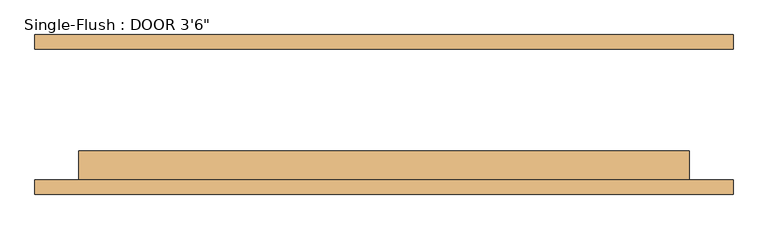
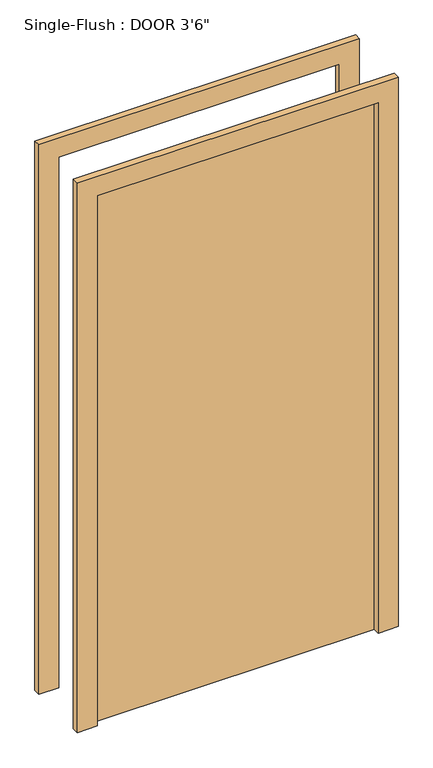
"""IFC4 building model written with IfcOpenShell, lengths in millimetres: door geometry."""

from ifc_helpers import new_model, si_unit, frame, origin, origin_with_axes, place, context, project, spatial, polyline, outline, extrude, source, transform, mapped, element, save


def door_0848dd25(model_context):
    return source(origin(), model_context, "Body", "SweptSolid", [
        extrude(outline(polyline([(2209.8, -609.6), (0.0, -609.6), (0.0, -533.4), (2133.6, -533.4), (2133.6, 533.4), (0.0, 533.4), (0.0, 609.6), (2209.8, 609.6), (2209.8, -609.6)])), frame((0.0, -139.7, 0.0), z_axis=(0.0, 1.0, 0.0), x_axis=(0.0, 0.0, 1.0)), (0.0, 0.0, 1.0), 25.4),
        extrude(outline(polyline([(2209.8, 609.6), (2209.8, -609.6), (0.0, -609.6), (0.0, -533.4), (2133.6, -533.4), (2133.6, 533.4), (0.0, 533.4), (0.0, 609.6), (2209.8, 609.6)])), frame((0.0, 114.3, 0.0), z_axis=(0.0, 1.0, 0.0), x_axis=(0.0, 0.0, 1.0)), (0.0, 0.0, 1.0), 25.4),
        extrude(outline(polyline([(533.4, -63.5), (533.4, -114.3), (-533.4, -114.3), (-533.4, -63.5), (533.4, -63.5)])), origin_with_axes(), (0.0, 0.0, 1.0), 2133.6),
    ])


if __name__ == "__main__":
    model = new_model("IFC4")
    model_context = context("Model", 3, world=origin())
    ifc_project = project(units=[si_unit("LENGTHUNIT", "METRE", prefix="MILLI")], contexts=[model_context])
    site = spatial("IfcSite", under=ifc_project)
    building = spatial("IfcBuilding", under=site)
    placement = place(None, origin())
    door_shape = door_0848dd25(model_context)
    element("IfcDoor", 1, ObjectType="Single-Flush : DOOR 3'6\"", at=placement, inside=building, context=model_context, shape_type="MappedRepresentation", body=[
        mapped(door_shape, transform((0.0, 0.0, 0.0), x_axis=(1.0, 0.0, 0.0), y_axis=(0.0, 1.0, 0.0), z_axis=(0.0, 0.0, 1.0))),
    ])
    save(model, "model.ifc")

# Revit data of these elements
# Type "Single-Flush : DOOR 3'6\""
#   Type Mark = "9"
#   Construction Type Id = "MDOOR"
#   Assembly Code = "C1020"
#   Analytic Construction = "Metal"
#   Thickness = 0' - 2"
#   Heat Transfer Coefficient (U) = 0.651978 BTU/(h·ft²·°F)
#   Height = 7' - 0"
#   Trim Projection Ext = 0' - 1"
#   Trim Projection Int = 0' - 1"
#   Trim Width = 0' - 3"
#   Width = 3' - 6"
#   Define Thermal Properties by = 1
#   Door Material = Door - Panel
#   Frame Material = Door - Frame
#   Visual Light Transmittance = 0
#   Solar Heat Gain Coefficient = 0
#   Function = (empty or 0)
#   Wall Closure = (empty or 0)
# Element 1 (IfcDoor, "Single-Flush : DOOR 3'6\"")
#   Materials on its faces: "Door - Frame", "Door - Panel"
# Materials
#   "Door - Panel": class "Wood", colour RGB 210 159 95, transparency 0, Cost = 0
#   "Door - Frame": colour RGB 118 70 51, transparency 0, Cost = 0
